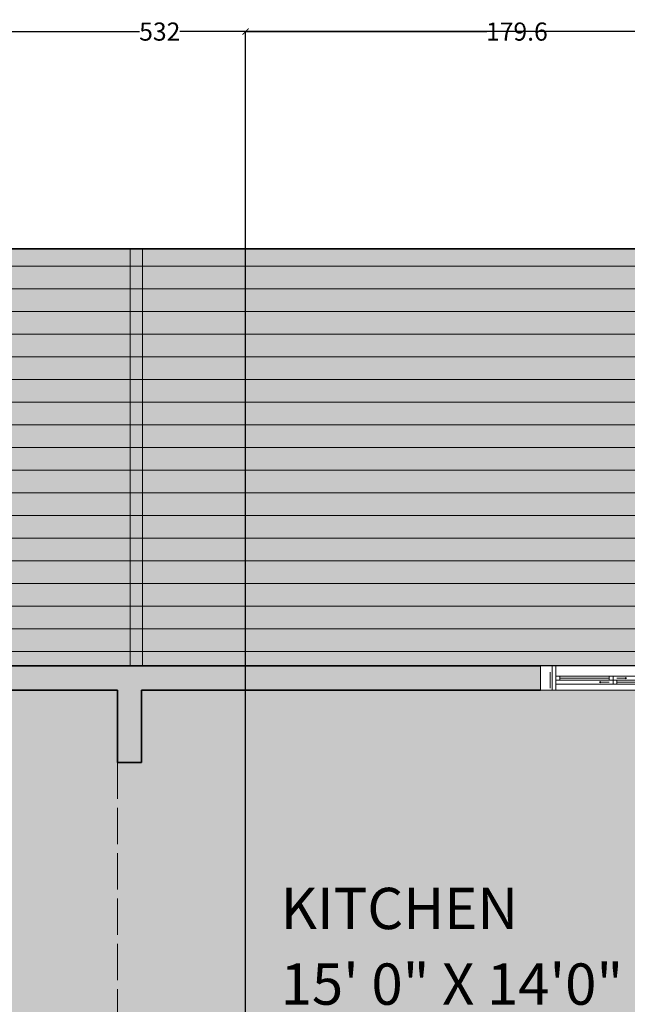
# Model space of a CAD drawing. Units: inches. Extents: x 1704 to 6393, y -157 to 1172.
# Tile 89 of 122: x 2293 to 2494, y 783 to 1109. Entities that reach past the tile are written whole.
import ezdxf

# ---------------------------------------------------------------- set-up
doc = ezdxf.new("R2010")
doc.units = ezdxf.units.IN
doc.header["$MEASUREMENT"] = 0
doc.linetypes.add('ACAD_ISO02W100', pattern=[15, 12, -3])
for name, color, linetype, lineweight in [('A-ANNO-DIMS', 7, 'Continuous', 13), ('A-AREA-IDEN', 7, 'Continuous', 18), ('A-WALL-OVHD', 8, 'ACAD_ISO02W100', 13), ('A-WALL-PATT', 7, 'Continuous', 13), ('C-PROP', 7, 'Continuous', 35), ('L-DECK-PLNK-PATT', 250, 'Continuous', 13), ('L-HRDS', 8, 'Continuous', 18), ('WALLS', 7, 'Continuous', 35), ('WINDOWS', 2, 'Continuous', 18)]:
    doc.layers.add(name, color=color, linetype=linetype, lineweight=lineweight)
doc.layers.add('A-FLOR-PATT', color=7, linetype='Continuous', lineweight=13, true_color=0xf2f2f2)
doc.layers.add('L-DECK-PATT', color=35, linetype='Continuous', lineweight=13, true_color=0xa6725b)
doc.styles.get("Standard").update_dxf_attribs({"font": 'arial.ttf'})
doc.dimstyles.get("Standard").update_dxf_attribs({"dimtxt": 6, "dimasz": 2, "dimexe": 0.18, "dimexo": 0.0625, "dimgap": 0.09, "dimtad": 0, "dimtih": 1, "dimtoh": 1, "dimdec": 1, "dimzin": 0, "dimdsep": 46, "dimlunit": 3, "dimtxsty": 'Standard', "dimblk": 'ARCHTICK', "dimcen": 0.09, "dimadec": 0, "dimazin": 0, "dimtfac": 1, "dimtdec": 1, "dimtofl": 0, "dimtmove": 0, "dimatfit": 3, "dimfxl": 1, "dimtolj": 1, "dimtzin": 0, "dimarcsym": 0})

# ---------------------------------------------------------------- blocks, each defined once
blk = doc.blocks.new('WIN-SLIDER-48')
for p, q in [((3.83, 8), (0, 8)), ((5.13, 8), (42.87, 8)), ((44.17, 8), (48, 8)), ((3.18, 5.86), (3.18, 0.65)), ((6.43, 4.55), (22.7, 4.55)), ((6.43, 3.9), (22.7, 3.9)), ((24, 4.55), (42.87, 4.55)), ((25.3, 3.9), (28.1, 3.9)), ((44.82, 5.86), (44.82, 0.65)), ((24, 1.95), (5.13, 1.95)), ((6.43, 3.25), (22.7, 3.25)), ((22.7, 2.6), (19.9, 2.6)), ((25.3, 3.25), (41.56, 3.25)), ((25.3, 2.6), (41.56, 2.6)), ((25.3, 1.95), (41.56, 1.95)), ((3.83, 0), (0, 0)), ((5.13, 0), (42.87, 0)), ((44.17, 0), (48, 0))]:
    blk.add_line(p, q)
for points in [[(5.13, 0), (3.83, 0), (3.83, 8), (5.13, 8)], [(42.87, 0), (44.17, 0), (44.17, 8), (42.87, 8)], [(5.13, 3.25), (6.43, 3.25), (6.43, 4.55), (5.13, 4.55)], [(22.7, 3.25), (24, 3.25), (24, 4.55), (22.7, 4.55)], [(28.43, 3.9), (28.1, 4.1), (28.1, 3.71)], [(19.57, 2.6), (19.9, 2.8), (19.9, 2.41)], [(24, 1.95), (25.3, 1.95), (25.3, 3.25), (24, 3.25)], [(41.56, 1.95), (42.87, 1.95), (42.87, 3.25), (41.56, 3.25)]]:
    blk.add_lwpolyline(points, close=True)
blk = doc.blocks.new('_ArchTick')
at = {"color": 0, "linetype": 'ByBlock', "const_width": 0.15}
blk.add_lwpolyline([(-0.5, -0.5), (0.5, 0.5)], dxfattribs=at)
blk = doc.blocks.new('*D92')
at = {"layer": 'A-ANNO-DIMS', "color": 0, "lineweight": -2, "transparency": 16777216}
for p, q in [((2073.35, 895.28), (2073.35, 1105.29)), ((2073.35, 1105.11), (2332.66, 1105.11)), ((2605.35, 1105.11), (2346.04, 1105.11)), ((2605.35, 895.28), (2605.35, 1105.29))]:
    blk.add_line(p, q, dxfattribs=at)
at = {"layer": 'Defpoints', "color": 0, "lineweight": -3, "transparency": 16777216}
for p in [(2605.35, 1105.11), (2073.35, 895.21), (2605.35, 895.21)]:
    blk.add_point(p, dxfattribs=at)
at = {"layer": 'A-ANNO-DIMS', "color": 0, "lineweight": -2, "transparency": 16777216, "xscale": 2, "yscale": 2, "zscale": 2, "rotation": 180}
blk.add_blockref('_ArchTick', (2073.35, 1105.11), dxfattribs=at)
at = {"layer": 'A-ANNO-DIMS', "color": 0, "lineweight": -2, "transparency": 16777216, "xscale": 2, "yscale": 2, "zscale": 2}
blk.add_blockref('_ArchTick', (2605.35, 1105.11), dxfattribs=at)
at = {"layer": 'A-ANNO-DIMS', "color": 0, "transparency": 16777216, "insert": (2339.35, 1105.11), "char_height": 6, "attachment_point": 5}
blk.add_mtext('\\A1;532', dxfattribs=at)
blk = doc.blocks.new('*D93')
at = {"layer": 'A-ANNO-DIMS', "color": 0, "lineweight": -2, "transparency": 16777216}
for p, q in [((2605.29, 895.21), (1829.7, 895.21)), ((1829.88, 895.21), (1829.88, 495.87)), ((1829.88, 90.21), (1829.88, 489.56)), ((2605.29, 90.21), (1829.7, 90.21))]:
    blk.add_line(p, q, dxfattribs=at)
at = {"layer": 'Defpoints', "color": 0, "lineweight": -3, "transparency": 16777216}
for p in [(2605.35, 895.21), (1829.88, 90.21), (2605.35, 90.21)]:
    blk.add_point(p, dxfattribs=at)
at = {"layer": 'A-ANNO-DIMS', "color": 0, "lineweight": -2, "transparency": 16777216, "xscale": 2, "yscale": 2, "zscale": 2}
for p, rotation in [((1829.88, 895.21), 90), ((1829.88, 90.21), 270)]:
    blk.add_blockref('_ArchTick', p, dxfattribs=dict(at, rotation=rotation))
at = {"layer": 'A-ANNO-DIMS', "color": 0, "transparency": 16777216, "insert": (1829.88, 492.71), "char_height": 6, "attachment_point": 5}
blk.add_mtext('\\A1;805', dxfattribs=at)
blk = doc.blocks.new('*D102')
at = {"layer": 'A-ANNO-DIMS', "color": 0, "lineweight": -2, "transparency": 16777216}
for p, q in [((2367.74, 711.28), (2367.74, 1105.29)), ((2367.74, 1105.11), (2447.61, 1105.11)), ((2547.35, 1105.11), (2467.47, 1105.11)), ((2547.35, 711.28), (2547.35, 1105.29))]:
    blk.add_line(p, q, dxfattribs=at)
at = {"layer": 'Defpoints', "color": 0, "lineweight": -3, "transparency": 16777216}
for p in [(2547.35, 1105.11), (2367.74, 711.21), (2547.35, 711.21)]:
    blk.add_point(p, dxfattribs=at)
at = {"layer": 'A-ANNO-DIMS', "color": 0, "lineweight": -2, "transparency": 16777216, "xscale": 2, "yscale": 2, "zscale": 2, "rotation": 180}
blk.add_blockref('_ArchTick', (2367.74, 1105.11), dxfattribs=at)
at = {"layer": 'A-ANNO-DIMS', "color": 0, "lineweight": -2, "transparency": 16777216, "xscale": 2, "yscale": 2, "zscale": 2}
blk.add_blockref('_ArchTick', (2547.35, 1105.11), dxfattribs=at)
at = {"layer": 'A-ANNO-DIMS', "color": 0, "transparency": 16777216, "insert": (2457.54, 1105.11), "char_height": 6, "attachment_point": 5}
blk.add_mtext('\\A1;179.6', dxfattribs=at)

msp = doc.modelspace()

# ---------------------------------------------------------------- hatches: boundary and pattern name
at = {"layer": 'A-FLOR-PATT', "transparency": 33554528}
h = msp.add_hatch(color=256, dxfattribs=at)
h.dxf.hatch_style = 1
h.paths.add_polyline_path([(2325.349, 863.213), (2325.349, 887.213), (2263.349, 887.213), (2167.349, 887.213), (2081.349, 887.213), (2081.349, 719.213), (2277.349, 719.213), (2277.349, 711.213), (2277.349, 372.213), (2349.349, 372.213), (2381.349, 372.213), (2381.349, 364.213), (2353.349, 364.213), (2353.349, 270.213), (2381.349, 270.213), (2381.349, 266.213), (2357.349, 266.213), (2357.349, 98.213), (2381.349, 98.213), (2385.181, 98.213), (2386.482, 98.213), (2424.215, 98.213), (2425.516, 98.213), (2429.349, 98.213), (2597.349, 98.213), (2597.349, 146.213), (2597.349, 218.213), (2597.349, 266.213), (2423.349, 266.213), (2423.349, 270.213), (2473.349, 270.213), (2473.349, 294.213), (2477.349, 294.213), (2477.349, 270.213), (2547.349, 270.213), (2547.349, 364.213), (2477.349, 364.213), (2477.349, 318.213), (2473.349, 318.213), (2473.349, 364.213), (2423.349, 364.213), (2423.349, 372.213), (2469.349, 372.213), (2469.349, 459.213), (2469.349, 538.213), (2350.349, 538.213), (2350.349, 565.713), (2358.349, 565.713), (2358.349, 545.213), (2420.349, 545.213), (2420.349, 610.213), (2358.349, 610.213), (2358.349, 589.713), (2350.349, 589.713), (2350.349, 615.213), (2425.349, 615.213), (2425.349, 607.213), (2425.349, 546.213), (2469.349, 546.213), (2514.349, 546.213), (2514.349, 607.213), (2449.349, 607.213), (2449.349, 615.213), (2451.738, 615.213), (2451.738, 659.213), (2427.738, 659.213), (2427.738, 665.213), (2367.738, 665.213), (2367.738, 667.213), (2367.738, 711.213), (2325.349, 711.213), (2325.349, 719.213), (2325.349, 755.213), (2325.349, 763.213)])
h.paths.add_polyline_path([(2233.858, 822.533, -0.187247), (2233.858, 809.14), (2231.697, 808.804, 0.0848928), (2233.131, 814.486), (2230.424, 814.486, -0.1042581), (2228.553, 808.313), (2217.751, 807.156, -0.2222222), (2217.751, 824.517), (2228.553, 823.359, -0.1042581), (2230.424, 817.186), (2233.131, 817.186, 0.0848928), (2231.697, 822.868)], flags=16)
h.paths.add_polyline_path([(2213.621, 833.197), (2213.621, 798.475), (2156.048, 798.475), (2156.048, 833.197)], flags=16)
h.paths.add_polyline_path([(2203.932, 848.099), (2205.089, 837.296, -0.2222222), (2187.728, 837.296), (2188.885, 848.099, -0.1042581), (2195.058, 849.969), (2195.058, 852.676, 0.0848928), (2189.377, 851.242), (2189.712, 853.404, -0.187247), (2203.105, 853.404), (2203.44, 851.242, 0.0848928), (2197.759, 852.676), (2197.759, 849.969, -0.1042581)], flags=16)
h.paths.add_polyline_path([(2181.941, 837.296, -0.2222222), (2164.58, 837.296), (2165.737, 848.099, -0.1042581), (2171.91, 849.969), (2171.91, 852.676, 0.0848928), (2166.229, 851.242), (2166.564, 853.404, -0.187247), (2179.957, 853.404), (2180.292, 851.242, 0.0848928), (2174.611, 852.676), (2174.611, 849.969, -0.1042581), (2180.784, 848.099)], flags=16)
h.paths.add_polyline_path([(2205.089, 794.376), (2203.932, 783.574, -0.1042581), (2197.759, 781.703), (2197.759, 778.996, 0.0848928), (2203.44, 780.43), (2203.105, 778.269, -0.187247), (2189.712, 778.269), (2189.377, 780.43, 0.0848928), (2195.058, 778.996), (2195.058, 781.703, -0.1042581), (2188.885, 783.574), (2187.728, 794.376, -0.2222222)], flags=16)
h.paths.add_polyline_path([(2181.941, 794.376), (2180.784, 783.574, -0.1042581), (2174.611, 781.703), (2174.611, 778.996, 0.0848928), (2180.292, 780.43), (2179.957, 778.269, -0.187247), (2166.564, 778.269), (2166.229, 780.43, 0.0848928), (2171.91, 778.996), (2171.91, 781.703, -0.1042581), (2165.737, 783.574), (2164.58, 794.376, -0.2222222)], flags=16)
h.paths.add_polyline_path([(2151.918, 807.156), (2141.116, 808.313, -0.1042581), (2139.245, 814.486), (2136.539, 814.486, 0.0848928), (2137.972, 808.804), (2135.811, 809.14, -0.187247), (2135.811, 822.533), (2137.972, 822.868, 0.0848928), (2136.539, 817.186), (2139.245, 817.186, -0.1042581), (2141.116, 823.359), (2151.918, 824.517, -0.2222222)], flags=16)
h.paths.add_polyline_path([(2357.868, 363.41), (2358.814, 363.41, 0.7537605)], flags=16)
h.paths.add_polyline_path([(2372.241, 363.117), (2372.248, 363.117), (2372.248, 363.343), (2371.302, 363.343), (2371.302, 363.139, -1.3603913)], flags=16)
h.paths.add_polyline_path([(2371.309, 272.716), (2371.302, 272.716), (2371.302, 272.49), (2372.248, 272.49), (2372.248, 272.693, -1.3603913)], flags=16)
h.paths.add_polyline_path([(2357.875, 272.716), (2357.868, 272.716), (2357.868, 272.49), (2358.814, 272.49), (2358.814, 272.693, -1.3603913)], flags=16)
h.paths.add_polyline_path([(2353.769, 363.074), (2376.347, 363.074), (2376.347, 272.759), (2353.769, 272.759)], flags=16)
h.paths.add_polyline_path([(2354.772, 362.07), (2375.344, 362.07), (2375.344, 273.762), (2354.772, 273.762)], flags=0)
h.paths.add_polyline_path([(2357.868, 363.343), (2358.814, 363.343), (2358.814, 363.117), (2357.868, 363.117)], flags=16)
h.paths.add_polyline_path([(2359.288, 359.184), (2359.288, 360.063), (2370.828, 360.063), (2370.828, 359.184), (2374.332, 359.184), (2374.332, 358.464), (2372.835, 358.464), (2372.835, 357.541), (2374.332, 357.541), (2374.332, 356.82), (2372.835, 356.82), (2372.835, 355.898), (2374.332, 355.898), (2374.332, 355.177), (2372.835, 355.177), (2372.835, 354.254), (2374.332, 354.254), (2374.332, 353.534), (2372.835, 353.534), (2372.835, 352.611), (2374.332, 352.611), (2374.332, 351.89), (2372.835, 351.89), (2372.835, 350.968), (2374.332, 350.968), (2374.332, 350.247), (2372.835, 350.247), (2372.835, 349.324), (2374.332, 349.324), (2374.332, 348.604), (2372.835, 348.604), (2372.835, 347.681), (2374.332, 347.681), (2374.332, 346.96), (2372.835, 346.96), (2372.835, 346.038), (2374.332, 346.038), (2374.332, 345.317), (2372.835, 345.317), (2372.835, 344.395), (2374.332, 344.395), (2374.332, 343.674), (2372.835, 343.674), (2372.835, 342.751), (2374.332, 342.751), (2374.332, 342.03), (2372.835, 342.03), (2372.835, 341.108), (2374.332, 341.108), (2374.332, 340.387), (2372.835, 340.387), (2372.835, 339.465), (2374.332, 339.465), (2374.332, 338.744), (2372.835, 338.744), (2372.835, 337.821), (2374.332, 337.821), (2374.332, 337.1), (2372.835, 337.1), (2372.835, 336.178), (2374.332, 336.178), (2374.332, 335.457), (2372.835, 335.457), (2372.835, 334.535), (2374.332, 334.535), (2374.332, 333.814), (2372.835, 333.814), (2372.835, 332.891), (2374.332, 332.891), (2374.332, 332.171), (2372.835, 332.171), (2372.835, 331.248), (2374.332, 331.248), (2374.332, 330.527), (2372.835, 330.527), (2372.835, 329.605), (2374.332, 329.605), (2374.332, 328.884), (2372.835, 328.884), (2372.835, 327.961), (2374.332, 327.961), (2374.332, 327.241), (2372.835, 327.241), (2372.835, 326.318), (2374.332, 326.318), (2374.332, 325.597), (2372.835, 325.597), (2372.835, 324.675), (2374.332, 324.675), (2374.332, 323.954), (2372.835, 323.954), (2372.835, 323.031), (2374.332, 323.031), (2374.332, 322.311), (2372.835, 322.311), (2372.835, 321.388), (2374.332, 321.388), (2374.332, 320.667), (2372.835, 320.667), (2372.835, 319.745), (2374.332, 319.745), (2374.332, 319.024), (2372.835, 319.024), (2372.835, 318.102), (2374.332, 318.102), (2374.332, 317.381), (2372.835, 317.381), (2372.835, 316.458), (2374.332, 316.458), (2374.332, 315.737), (2372.835, 315.737), (2372.835, 314.815), (2374.332, 314.815), (2374.332, 314.094), (2372.835, 314.094), (2372.835, 313.172), (2374.332, 313.172), (2374.332, 312.451), (2372.835, 312.451), (2372.835, 311.528), (2374.332, 311.528), (2374.332, 310.807), (2372.835, 310.807), (2372.835, 309.885), (2374.332, 309.885), (2374.332, 309.164), (2372.835, 309.164), (2372.835, 308.242), (2374.332, 308.242), (2374.332, 307.521), (2372.835, 307.521), (2372.835, 306.598), (2374.332, 306.598), (2374.332, 305.878), (2372.835, 305.878), (2372.835, 304.955), (2374.332, 304.955), (2374.332, 304.234), (2372.835, 304.234), (2372.835, 303.312), (2374.332, 303.312), (2374.332, 302.591), (2372.835, 302.591), (2372.835, 301.668), (2374.332, 301.668), (2374.332, 300.948), (2372.835, 300.948), (2372.835, 300.025), (2374.332, 300.025), (2374.332, 299.304), (2372.835, 299.304), (2372.835, 298.382), (2374.332, 298.382), (2374.332, 297.661), (2372.835, 297.661), (2372.835, 296.738), (2374.332, 296.738), (2374.332, 296.018), (2372.835, 296.018), (2372.835, 295.095), (2374.332, 295.095), (2374.332, 294.374), (2372.835, 294.374), (2372.835, 293.452), (2374.332, 293.452), (2374.332, 292.731), (2372.835, 292.731), (2372.835, 291.809), (2374.332, 291.809), (2374.332, 291.088), (2372.835, 291.088), (2372.835, 290.165), (2374.332, 290.165), (2374.332, 289.444), (2372.835, 289.444), (2372.835, 288.522), (2374.332, 288.522), (2374.332, 287.801), (2372.835, 287.801), (2372.835, 286.879), (2374.332, 286.879), (2374.332, 286.158), (2372.835, 286.158), (2372.835, 285.235), (2374.332, 285.235), (2374.332, 284.514), (2372.835, 284.514), (2372.835, 283.592), (2374.332, 283.592), (2374.332, 282.871), (2372.835, 282.871), (2372.835, 281.949), (2374.332, 281.949), (2374.332, 281.228), (2372.835, 281.228), (2372.835, 280.305), (2374.332, 280.305), (2374.332, 279.585), (2372.835, 279.585), (2372.835, 278.662), (2374.332, 278.662), (2374.332, 277.941), (2372.835, 277.941), (2372.835, 277.019), (2374.332, 277.019), (2374.332, 276.298), (2370.828, 276.298), (2370.828, 275.769), (2359.288, 275.769), (2359.288, 276.298), (2355.784, 276.298), (2355.784, 277.019), (2357.281, 277.019), (2357.281, 277.941), (2355.784, 277.941), (2355.784, 278.662), (2357.281, 278.662), (2357.281, 279.585), (2355.784, 279.585), (2355.784, 280.305), (2357.281, 280.305), (2357.281, 281.228), (2355.784, 281.228), (2355.784, 281.949), (2357.281, 281.949), (2357.281, 282.871), (2355.784, 282.871), (2355.784, 283.592), (2357.281, 283.592), (2357.281, 284.514), (2355.784, 284.514), (2355.784, 285.235), (2357.281, 285.235), (2357.281, 286.158), (2355.784, 286.158), (2355.784, 286.879), (2357.281, 286.879), (2357.281, 287.801), (2355.784, 287.801), (2355.784, 288.522), (2357.281, 288.522), (2357.281, 289.444), (2355.784, 289.444), (2355.784, 290.165), (2357.281, 290.165), (2357.281, 291.088), (2355.784, 291.088), (2355.784, 291.809), (2357.281, 291.809), (2357.281, 292.731), (2355.784, 292.731), (2355.784, 293.452), (2357.281, 293.452), (2357.281, 294.374), (2355.784, 294.374), (2355.784, 295.095), (2357.281, 295.095), (2357.281, 296.018), (2355.784, 296.018), (2355.784, 296.738), (2357.281, 296.738), (2357.281, 297.661), (2355.784, 297.661), (2355.784, 298.382), (2357.281, 298.382), (2357.281, 299.304), (2355.784, 299.304), (2355.784, 300.025), (2357.281, 300.025), (2357.281, 300.948), (2355.784, 300.948), (2355.784, 301.668), (2357.281, 301.668), (2357.281, 302.591), (2355.784, 302.591), (2355.784, 303.312), (2357.281, 303.312), (2357.281, 304.234), (2355.784, 304.234), (2355.784, 304.955), (2357.281, 304.955), (2357.281, 305.878), (2355.784, 305.878), (2355.784, 306.598), (2357.281, 306.598), (2357.281, 307.521), (2355.784, 307.521), (2355.784, 308.242), (2357.281, 308.242), (2357.281, 309.164), (2355.784, 309.164), (2355.784, 309.885), (2357.281, 309.885), (2357.281, 310.807), (2355.784, 310.807), (2355.784, 311.528), (2357.281, 311.528), (2357.281, 312.451), (2355.784, 312.451), (2355.784, 313.172), (2357.281, 313.172), (2357.281, 314.094), (2355.784, 314.094), (2355.784, 314.815), (2357.281, 314.815), (2357.281, 315.737), (2355.784, 315.737), (2355.784, 316.458), (2357.281, 316.458), (2357.281, 317.381), (2355.784, 317.381), (2355.784, 318.102), (2357.281, 318.102), (2357.281, 319.024), (2355.784, 319.024), (2355.784, 319.745), (2357.281, 319.745), (2357.281, 320.667), (2355.784, 320.667), (2355.784, 321.388), (2357.281, 321.388), (2357.281, 322.311), (2355.784, 322.311), (2355.784, 323.031), (2357.281, 323.031), (2357.281, 323.954), (2355.784, 323.954), (2355.784, 324.675), (2357.281, 324.675), (2357.281, 325.597), (2355.784, 325.597), (2355.784, 326.318), (2357.281, 326.318), (2357.281, 327.241), (2355.784, 327.241), (2355.784, 327.961), (2357.281, 327.961), (2357.281, 328.884), (2355.784, 328.884), (2355.784, 329.605), (2357.281, 329.605), (2357.281, 330.527), (2355.784, 330.527), (2355.784, 331.248), (2357.281, 331.248), (2357.281, 332.171), (2355.784, 332.171), (2355.784, 332.891), (2357.281, 332.891), (2357.281, 333.814), (2355.784, 333.814), (2355.784, 334.535), (2357.281, 334.535), (2357.281, 335.457), (2355.784, 335.457), (2355.784, 336.178), (2357.281, 336.178), (2357.281, 337.1), (2355.784, 337.1), (2355.784, 337.821), (2357.281, 337.821), (2357.281, 338.744), (2355.784, 338.744), (2355.784, 339.465), (2357.281, 339.465), (2357.281, 340.387), (2355.784, 340.387), (2355.784, 341.108), (2357.281, 341.108), (2357.281, 342.03), (2355.784, 342.03), (2355.784, 342.751), (2357.281, 342.751), (2357.281, 343.674), (2355.784, 343.674), (2355.784, 344.395), (2357.281, 344.395), (2357.281, 345.317), (2355.784, 345.317), (2355.784, 346.038), (2357.281, 346.038), (2357.281, 346.96), (2355.784, 346.96), (2355.784, 347.681), (2357.281, 347.681), (2357.281, 348.604), (2355.784, 348.604), (2355.784, 349.324), (2357.281, 349.324), (2357.281, 350.247), (2355.784, 350.247), (2355.784, 350.968), (2357.281, 350.968), (2357.281, 351.89), (2355.784, 351.89), (2355.784, 352.611), (2357.281, 352.611), (2357.281, 353.534), (2355.784, 353.534), (2355.784, 354.254), (2357.281, 354.254), (2357.281, 355.177), (2355.784, 355.177), (2355.784, 355.898), (2357.281, 355.898), (2357.281, 356.82), (2355.784, 356.82), (2355.784, 357.541), (2357.281, 357.541), (2357.281, 358.464), (2355.784, 358.464), (2355.784, 359.184)], flags=0)
h = msp.add_hatch(color=256, dxfattribs=at)
h.dxf.hatch_style = 1
h.paths.add_polyline_path([(2517.349, 861.213), (2513.349, 861.213), (2513.349, 887.213), (2509.516, 887.213), (2508.215, 887.213), (2470.482, 887.213), (2469.181, 887.213), (2465.349, 887.213), (2333.349, 887.213), (2333.349, 863.213), (2325.349, 863.213), (2325.349, 763.213), (2365.349, 763.213), (2365.349, 719.213), (2513.349, 719.213), (2513.349, 753.213), (2515.349, 753.213), (2500.349, 779.194), (2501.431, 779.819), (2501.444, 779.796, -0.1041754), (2513.349, 783.146), (2513.349, 813.213), (2517.349, 813.213)])
h.paths.add_polyline_path([(2597.349, 818.213), (2601.349, 818.213), (2600.05, 818.963), (2618.034, 850.113, 0.1210664), (2601.349, 854.213), (2597.349, 854.213), (2597.349, 887.213), (2581.349, 887.213), (2533.349, 887.213), (2517.349, 887.213), (2517.349, 861.213), (2517.349, 813.213), (2517.349, 787.213), (2597.349, 787.213)])
h.paths.add_polyline_path([(2597.349, 783.213), (2517.349, 783.213), (2515.349, 783.213, 0.1210664), (2501.444, 779.796), (2516.792, 753.213), (2517.349, 753.213), (2517.349, 719.213), (2597.349, 719.213)])
at = {"layer": 'A-WALL-PATT', "transparency": 33554643}
h = msp.add_hatch(color=256, dxfattribs=at)
h.dxf.hatch_style = 1
h.paths.add_polyline_path([(2167.349, 895.213), (2073.349, 895.213), (2073.349, 887.213), (2081.349, 887.213), (2167.349, 887.213)])
h.paths.add_polyline_path([(2465.349, 895.213), (2273.349, 895.213), (2273.349, 903.213), (2263.349, 903.213), (2263.349, 895.213), (2263.349, 887.213), (2325.349, 887.213), (2325.349, 863.213), (2333.349, 863.213), (2333.349, 887.213), (2465.349, 887.213)])
h.paths.add_polyline_path([(2533.349, 895.213), (2513.349, 895.213), (2513.349, 887.213), (2513.349, 861.213), (2517.349, 861.213), (2517.349, 887.213), (2533.349, 887.213)])
h.paths.add_polyline_path([(2605.349, 895.213), (2581.349, 895.213), (2581.349, 887.213), (2597.349, 887.213), (2597.349, 854.213), (2605.349, 854.213)])
h.paths.add_polyline_path([(2605.349, 752.213), (2629.349, 752.213), (2629.349, 716.213), (2605.349, 716.213), (2605.349, 712.213), (2719.349, 712.213), (2719.349, 716.213), (2631.349, 716.213), (2631.349, 754.213), (2605.349, 754.213), (2605.349, 794.213), (2597.349, 794.213), (2597.349, 787.213), (2517.349, 787.213), (2517.349, 813.213), (2513.349, 813.213), (2513.349, 783.213), (2517.349, 783.213), (2597.349, 783.213), (2597.349, 719.213), (2517.349, 719.213), (2517.349, 753.213), (2513.349, 753.213), (2513.349, 719.213), (2365.349, 719.213), (2365.349, 763.213), (2325.349, 763.213), (2325.349, 755.213), (2357.349, 755.213), (2357.349, 719.213), (2325.349, 719.213), (2325.349, 711.213), (2547.349, 711.213), (2547.349, 615.213), (2449.349, 615.213), (2449.349, 607.213), (2514.349, 607.213), (2514.349, 546.213), (2439.349, 546.213), (2425.349, 546.213), (2425.349, 607.213), (2425.349, 615.213), (2350.349, 615.213), (2350.349, 589.713), (2358.349, 589.713), (2358.349, 610.213), (2420.349, 610.213), (2420.349, 545.213), (2358.349, 545.213), (2358.349, 565.713), (2350.349, 565.713), (2350.349, 538.213), (2469.349, 538.213), (2469.349, 459.213), (2469.349, 372.213), (2423.349, 372.213), (2423.349, 364.213), (2473.349, 364.213), (2473.349, 318.213), (2477.349, 318.213), (2477.349, 364.213), (2547.349, 364.213), (2547.349, 352.213), (2549.349, 352.213), (2549.349, 364.213), (2597.349, 364.213), (2597.349, 328.213), (2549.349, 328.213), (2547.349, 328.213), (2547.349, 326.213), (2549.349, 326.213), (2597.349, 326.213), (2605.349, 326.213), (2605.349, 377.057), (2597.349, 377.057), (2597.349, 372.213), (2477.349, 372.213), (2477.349, 451.213), (2597.349, 451.213), (2605.349, 451.213), (2605.349, 459.213), (2597.349, 459.213), (2477.349, 459.213), (2477.349, 538.213), (2597.349, 538.213), (2597.349, 495.213), (2605.349, 495.213), (2605.349, 512.213), (2631.349, 512.213), (2631.349, 568.213), (2605.349, 568.213), (2605.349, 577.213), (2597.349, 577.213), (2597.349, 542.213), (2518.349, 542.213), (2518.349, 607.213), (2532.349, 607.213), (2605.349, 607.213), (2605.349, 615.213), (2597.349, 615.213), (2551.349, 615.213), (2551.349, 711.213), (2597.349, 711.213), (2597.349, 645.213), (2605.349, 645.213), (2605.349, 712.213), (2605.349, 716.213)])
h.paths.add_polyline_path([(2605.349, 566.213), (2629.349, 566.213), (2629.349, 514.213), (2605.349, 514.213)], flags=16)
h.paths.add_polyline_path([(2381.349, 372.213), (2349.349, 372.213), (2349.349, 202.213), (2337.349, 202.213), (2337.349, 194.213), (2349.349, 194.213), (2349.349, 90.213), (2349.349, 72.213), (2357.349, 72.213), (2357.349, 90.213), (2381.349, 90.213), (2381.349, 98.213), (2357.349, 98.213), (2357.349, 266.213), (2381.349, 266.213), (2381.349, 270.213), (2353.349, 270.213), (2353.349, 364.213), (2381.349, 364.213)])
h.paths.add_polyline_path([(2605.349, 302.213), (2597.349, 302.213), (2597.349, 270.213), (2477.349, 270.213), (2477.349, 294.213), (2473.349, 294.213), (2473.349, 270.213), (2423.349, 270.213), (2423.349, 266.213), (2597.349, 266.213), (2597.349, 218.213), (2605.349, 218.213)])
h.paths.add_polyline_path([(2605.349, 146.213), (2597.349, 146.213), (2597.349, 98.213), (2429.349, 98.213), (2429.349, 90.213), (2597.349, 90.213), (2597.349, 72.213), (2605.349, 72.213), (2605.349, 90.213)])
h.paths.add_polyline_path([(2225.349, 202.213), (2049.349, 202.213), (2049.349, 194.213), (2225.349, 194.213)])
h.paths.add_polyline_path([(2289.349, 202.213), (2277.349, 202.213), (2273.349, 202.213), (2269.516, 202.213), (2269.516, 194.213), (2273.349, 194.213), (2277.349, 194.213), (2289.349, 194.213)])
h.paths.add_polyline_path([(2273.349, 372.213), (2029.19, 372.213), (2029.19, 364.213), (2273.349, 364.213)])
h.paths.add_polyline_path([(2277.349, 545.213), (2213.349, 545.213), (2213.349, 573.213), (2205.349, 573.213), (2177.349, 573.213), (2177.349, 545.213), (2073.349, 545.213), (2073.349, 538.213), (2081.349, 538.213), (2277.349, 538.213)])
h.paths.add_polyline_path([(2181.349, 545.213), (2181.349, 569.213), (2205.349, 569.213), (2205.349, 545.213)], flags=16)
h.paths.add_polyline_path([(2277.349, 719.213), (2081.349, 719.213), (2073.349, 719.213), (2073.349, 711.213), (2154.575, 711.213), (2205.349, 711.213), (2205.349, 687.213), (2205.349, 629.213), (2213.349, 629.213), (2273.349, 629.213), (2273.349, 631.213), (2207.349, 631.213), (2207.349, 707.213), (2231.349, 707.213), (2231.349, 709.213), (2207.349, 709.213), (2207.349, 711.213), (2277.349, 711.213)])
at = {"layer": 'L-DECK-PATT', "transparency": 33554544}
h = msp.add_hatch(color=256, dxfattribs=at)
h.dxf.hatch_style = 1
h.paths.add_polyline_path([(2329.589, 1033.213), (2065.589, 1033.213), (2065.589, 895.213), (2167.349, 895.213), (2263.349, 895.213), (2263.349, 903.213), (2273.349, 903.213), (2273.349, 895.213), (2329.589, 895.213)])
h.paths.add_polyline_path([(2664.349, 1033.213), (2333.589, 1033.213), (2333.589, 895.213), (2465.349, 895.213), (2469.181, 895.213), (2470.482, 895.213), (2508.215, 895.213), (2509.516, 895.213), (2513.349, 895.213), (2533.349, 895.213), (2581.349, 895.213), (2605.349, 895.213), (2664.349, 895.213)])
h.paths.add_polyline_path([(2333.589, 1033.213), (2329.589, 1033.213), (2329.589, 895.213), (2333.589, 895.213)])
at = {"layer": 'L-DECK-PLNK-PATT'}
h = msp.add_hatch(dxfattribs=at)
h.set_pattern_fill('LINE', color=256, scale=60)
h.paths.add_polyline_path([(2329.589, 1033.213), (2065.589, 1033.213), (2065.589, 895.213), (2167.349, 895.213), (2263.349, 895.213), (2263.349, 903.213), (2273.349, 903.213), (2273.349, 895.213), (2329.589, 895.213)])
h.paths.add_polyline_path([(2664.349, 1033.213), (2333.589, 1033.213), (2333.589, 895.213), (2465.349, 895.213), (2469.181, 895.213), (2470.482, 895.213), (2508.215, 895.213), (2509.516, 895.213), (2513.349, 895.213), (2533.349, 895.213), (2581.349, 895.213), (2605.349, 895.213), (2664.349, 895.213)])
h.paths.add_polyline_path([(2333.589, 1033.213), (2329.589, 1033.213), (2329.589, 895.213), (2333.589, 895.213)])

# ---------------------------------------------------------------- linework, layer by layer
at = {"layer": 'A-WALL-OVHD'}
msp.add_line((2325.349, 863.213), (2325.349, 763.213), dxfattribs=at)
at = {"layer": 'C-PROP'}
msp.add_line((2723.349, 1033.213), (1898.349, 1033.213), dxfattribs=at)
at = {"layer": 'L-HRDS'}
for p, q in [((2329.589, 895.213), (2329.589, 1033.213)), ((2333.589, 895.213), (2333.589, 1033.213))]:
    msp.add_line(p, q, dxfattribs=at)
at = {"layer": 'WALLS'}
for p, q in [((2465.349, 895.213), (2273.349, 895.213)), ((2325.349, 887.213), (2263.349, 887.213)), ((2325.349, 863.213), (2325.349, 887.213)), ((2465.349, 887.213), (2333.349, 887.213)), ((2333.349, 863.213), (2333.349, 887.213)), ((2325.349, 863.213), (2333.349, 863.213))]:
    msp.add_line(p, q, dxfattribs=at)
at = {"layer": 'WINDOWS'}
msp.add_line((2465.349, 887.213), (2465.349, 895.213), dxfattribs=at)

# ---------------------------------------------------------------- block references
msp.add_blockref('WIN-SLIDER-48', (2465.349, 887.213), dxfattribs=at)

# ---------------------------------------------------------------- texts
at = {"layer": 'A-ANNO-DIMS'}
msp.add_text('15\' 0" X 14\'0"', height=13.6672, dxfattribs=at).set_placement((2379.353, 783.068))
at = {"layer": 'A-AREA-IDEN'}
msp.add_text('KITCHEN', height=13.6672, dxfattribs=at).set_placement((2379.353, 808.093))

# ---------------------------------------------------------------- dimensions: what is measured, and where the dimension line sits
at = {"layer": 'A-ANNO-DIMS'}
for base, p1, p2, override, picture, middle in [((2605.349, 1105.107), (2073.349, 895.213), (2605.349, 895.213), {"dimdec": 0, "dimlfac": 1, "dimrnd": 0, "dimzin": 0, "dimdsep": 46, "dimlunit": 2}, '*D92', (2339.349, 1105.107)), ((2547.349, 1105.107), (2367.738, 711.213), (2547.349, 711.213), {"dimdec": 1, "dimlfac": 1, "dimrnd": 0, "dimzin": 0, "dimdsep": 46, "dimlunit": 2}, '*D102', (2457.543, 1105.107))]:
    dim = msp.add_linear_dim(base=base, p1=p1, p2=p2, dimstyle='Standard', override=override, dxfattribs=at)
    dim.commit()
    dim.dimension.update_dxf_attribs({"geometry": picture, "text_midpoint": middle})
dim = msp.add_linear_dim(base=(1829.878, 90.213), p1=(2605.349, 895.213), p2=(2605.349, 90.213), angle=90, dimstyle='Standard', override={"dimdec": 0, "dimlfac": 1, "dimrnd": 0, "dimzin": 0, "dimdsep": 46, "dimlunit": 2}, dxfattribs=at)
dim.commit()
dim.dimension.update_dxf_attribs({"geometry": '*D93', "text_midpoint": (1829.878, 492.713)})

doc.saveas('drawing.dxf')
